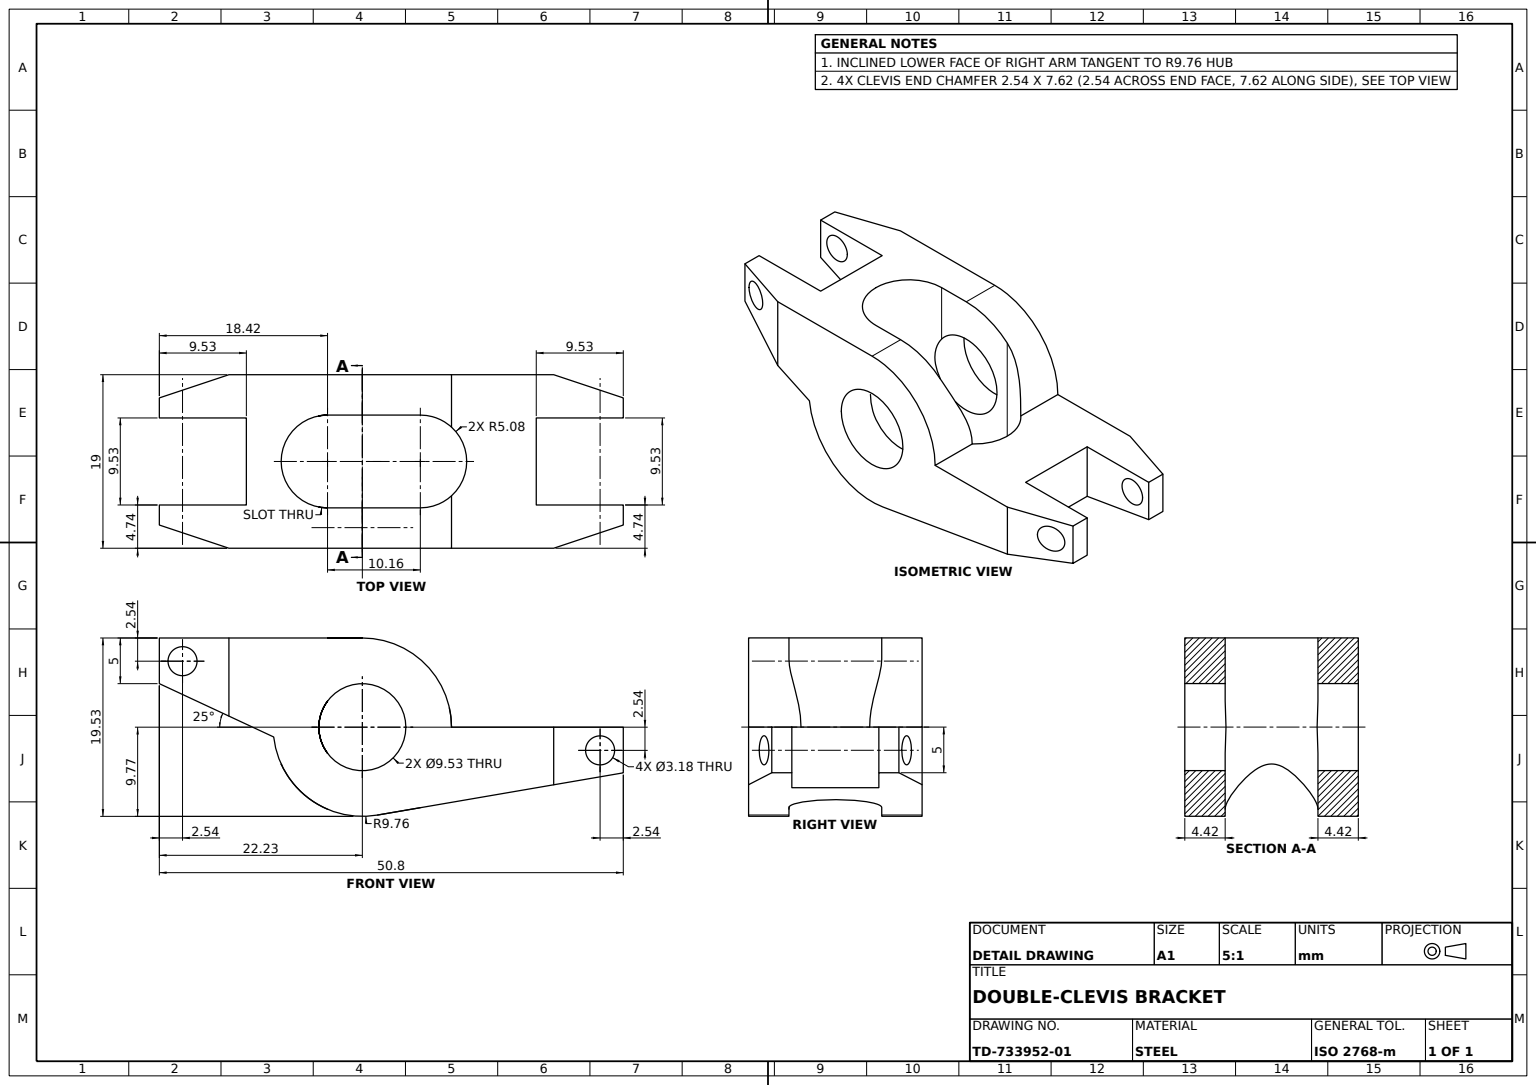
SolidWorks part; units mm, degrees
material "Plain Carbon Steel"
ref_plane "Front Plane" through (0, 0, 0) normal (0, 0, 1) x (1, 0, 0)
ref_plane "Top Plane" through (0, 0, 0) normal (0, 1, 0) x (1, 0, 0)
ref_plane "Right Plane" through (0, 0, 0) normal (1, 0, 0) x (0, 0, -1)
sketch "Rocker Arm Profile Sketch" plane through (0, 0, 0) normal (1, 0, 0) x (0, 0, -1)
  line L0 (0, 9.765) -> (-22.23, 9.765)
  line L1 (-22.23, 9.765) -> (-22.23, 4.765)
  line L2 (-22.23, 4.765) -> (-9.7056, -1.0752)
  line L3 (0, 0) -> (28.575, 0)
  line L4 (28.575, 0) -> (28.575, -5)
  line L5 (28.575, -5) -> (1.653, -9.6241)
  circle A0 centre (0, 0) radius 4.765
  arc A1 (-9.7056, -1.0752) -> (1.653, -9.6241) centre (0, 0) ccw
  arc A2 (9.765, 0) -> (0, 9.765) centre (0, 0) ccw
  circle A3 centre (0, 0) radius 9.765 construction
  point P7 (9.765, 0)
  dimension "D1" = 9.53
  dimension "D3" = 22.23
  dimension "D4" = 5
  dimension "D5" = 25
  dimension "D6" = 28.575
  dimension "D7" = 5
  dimension "D2" = 5
extrude "Rocker Arm Body" add sketch "Rocker Arm Profile Sketch" along normal mid plane 19
chamfer "End Chamfer 2.54x7.62" distance 2.54 distance2 7.62 2 edges at (9.5, 7.265, 22.23) (-9.5, -2.5, -28.575)
chamfer "End Chamfer 7.62x2.54" distance 7.62 distance2 2.54 2 edges at (-9.5, 7.265, 22.23) (9.5, -2.5, -28.575)
sketch "Hub Cut Sketch" plane through (0, 0, 0) normal (0, 1, 0) x (1, 0, 0)
  line L0 (0, -3.81) -> (0, 6.35) construction
  line L1 (-5.08, -3.81) -> (-5.08, 6.35)
  line L2 (5.08, -3.81) -> (5.08, 6.35)
  arc A0 (-5.08, -3.81) -> (5.08, -3.81) centre (0, -3.81) ccw
  arc A1 (5.08, 6.35) -> (-5.08, 6.35) centre (0, 6.35) ccw
  point P3 (0, 1.27)
  dimension "D1" = 10.16
  dimension "D2" = 10.16
  dimension "D3" = 3.81
extrude "Hub Cut" cut sketch "Hub Cut Sketch" against normal through all both and the other way through all
sketch "Fork Slot Sketch" plane through (0, 0, 0) normal (0, 1, 0) x (1, 0, 0)
  line L0 (6.96, -22.23) -> (-6.96, -22.23) construction
  line L1 (-4.765, 28.575) -> (4.765, 28.575)
  line L2 (-4.765, 28.575) -> (-4.765, 19.045)
  line L3 (-4.765, 19.045) -> (4.765, 19.045)
  line L4 (4.765, 28.575) -> (4.765, 19.045)
  line L5 (-4.765, 28.575) -> (4.765, 19.045) construction
  line L6 (-4.765, 19.045) -> (4.765, 28.575) construction
  line L7 (-4.765, -12.7) -> (4.765, -12.7)
  line L8 (-4.765, -12.7) -> (-4.765, -22.23)
  line L9 (-4.765, -22.23) -> (4.765, -22.23)
  line L10 (4.765, -12.7) -> (4.765, -22.23)
  line L11 (-4.765, -12.7) -> (4.765, -22.23) construction
  line L12 (-4.765, -22.23) -> (4.765, -12.7) construction
  line L13 (6.96, 28.575) -> (-6.96, 28.575) construction
  point P0 (0, 23.81)
  point P5 (0, -17.465)
  point P14 (0, 28.575)
  dimension "D1" = 9.53
  dimension "D2" = 9.53
  dimension "D3" = 9.53
  dimension "D4" = 9.53
extrude "Fork Slot Cut" cut sketch "Fork Slot Sketch" against normal through all both and the other way through all
sketch "Pin Holes Sketch" plane through (0, 0, 0) normal (1, 0, 0) x (0, 0, -1)
  line L0 (-22.23, 4.765) -> (-22.23, 9.765) construction
  line L1 (-22.23, 9.765) -> (-14.61, 9.765) construction
  line L2 (20.955, 0) -> (28.575, 0) construction
  line L3 (28.575, 0) -> (28.575, -5) construction
  circle A0 centre (-19.69, 7.225) radius 1.59
  circle A1 centre (26.035, -2.54) radius 1.59
  dimension "D1" = 3.18
  dimension "D2" = 2.54
  dimension "D3" = 2.54
  dimension "D4" = 2.54
  dimension "D5" = 2.54
extrude "Pin Holes 2xØ3.18" cut sketch "Pin Holes Sketch" against normal through all both and the other way through all
equation "\"3.815.2628044mm\"=5.2628"
